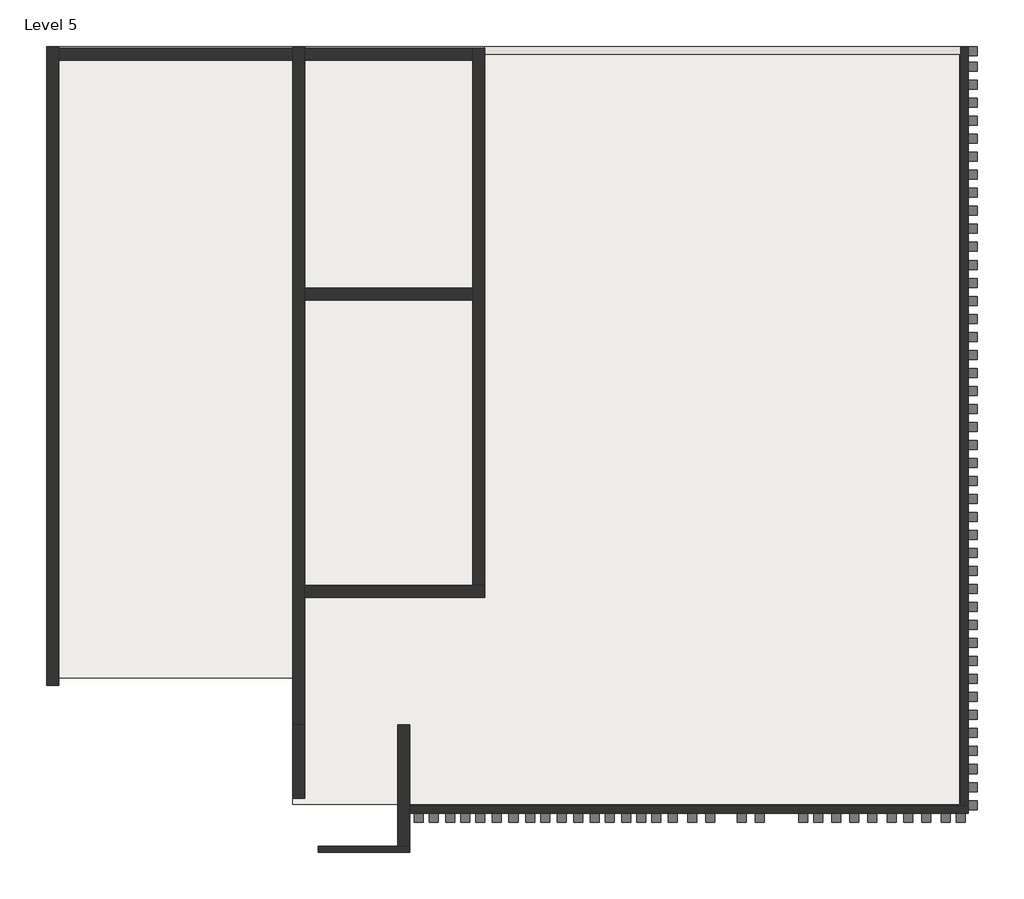
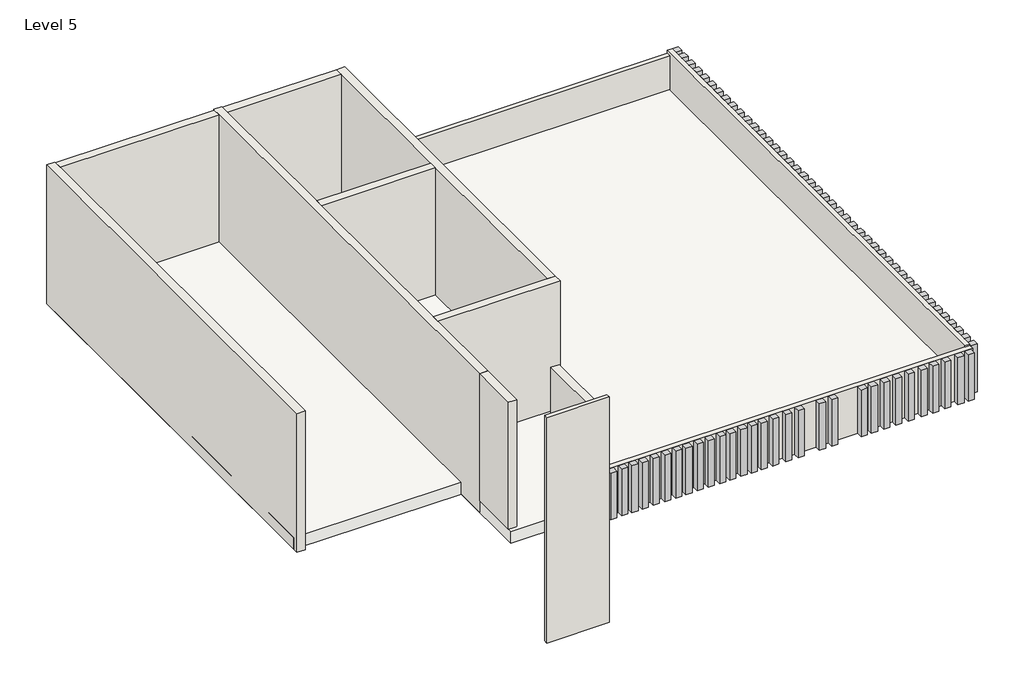
# One storey: 75 proxies, 12 walls, 1 roof.
"""IFC4 building model written with IfcOpenShell, lengths in millimetres."""

from ifc_helpers import new_model, si_unit, frame, origin, place, context, project, spatial, polyline, outline, extrude, faceted_brep, element, save

model = new_model("IFC4")

# Units and contexts
model_context = context("Model", 3, world=origin())
ifc_project = project(units=[si_unit("LENGTHUNIT", "METRE", prefix="MILLI")], contexts=[model_context])

# Site, building, storey
site = spatial("IfcSite", under=ifc_project)
building = spatial("IfcBuilding", under=site)
storey = spatial("IfcBuildingStorey", under=building, Name="Level 5", Elevation=14630.4)

# Proxies
placement = place(None, origin())
element("IfcBuildingElementProxy", 1, Name="Cornice", ObjectType="Cornice", at=placement, inside=storey, context=model_context, shape_type="SweptSolid", body=[
    extrude(outline(polyline([(-3003.9749149, -2254.9518013), (-3003.9749149, -2407.3518013), (-3156.3749149, -2407.3518013), (-3156.3749149, -2254.9518013), (-3003.9749149, -2254.9518013)])), frame((0.0, 0.0, 14630.4), z_axis=(0.0, 0.0, 1.0), x_axis=(1.0, 0.0, 0.0)), (0.0, 0.0, 1.0), 1229.0328786),
])
element("IfcBuildingElementProxy", 2, Name="Cornice", ObjectType="Cornice", at=placement, inside=storey, context=model_context, shape_type="SweptSolid", body=[
    extrude(outline(polyline([(-2749.9749149, -2254.9518013), (-2749.9749149, -2407.3518013), (-2902.3749149, -2407.3518013), (-2902.3749149, -2254.9518013), (-2749.9749149, -2254.9518013)])), frame((0.0, 0.0, 14630.4), z_axis=(0.0, 0.0, 1.0), x_axis=(1.0, 0.0, 0.0)), (0.0, 0.0, 1.0), 1229.0328786),
])
element("IfcBuildingElementProxy", 3, Name="Cornice", ObjectType="Cornice", at=placement, inside=storey, context=model_context, shape_type="SweptSolid", body=[
    extrude(outline(polyline([(-2470.5749149, -2254.9518013), (-2470.5749149, -2407.3518013), (-2622.9749149, -2407.3518013), (-2622.9749149, -2254.9518013), (-2470.5749149, -2254.9518013)])), frame((0.0, 0.0, 14630.4), z_axis=(0.0, 0.0, 1.0), x_axis=(1.0, 0.0, 0.0)), (0.0, 0.0, 1.0), 1229.0328786),
])
element("IfcBuildingElementProxy", 4, Name="Cornice", ObjectType="Cornice", at=placement, inside=storey, context=model_context, shape_type="SweptSolid", body=[
    extrude(outline(polyline([(-2216.5749149, -2254.9518013), (-2216.5749149, -2407.3518013), (-2368.9749149, -2407.3518013), (-2368.9749149, -2254.9518013), (-2216.5749149, -2254.9518013)])), frame((0.0, 0.0, 14630.4), z_axis=(0.0, 0.0, 1.0), x_axis=(1.0, 0.0, 0.0)), (0.0, 0.0, 1.0), 1229.0328786),
])
element("IfcBuildingElementProxy", 5, Name="Cornice", ObjectType="Cornice", at=placement, inside=storey, context=model_context, shape_type="SweptSolid", body=[
    extrude(outline(polyline([(-1962.5749149, -2254.9518013), (-1962.5749149, -2407.3518013), (-2114.9749149, -2407.3518013), (-2114.9749149, -2254.9518013), (-1962.5749149, -2254.9518013)])), frame((0.0, 0.0, 14630.4), z_axis=(0.0, 0.0, 1.0), x_axis=(1.0, 0.0, 0.0)), (0.0, 0.0, 1.0), 1229.0328786),
])
element("IfcBuildingElementProxy", 6, Name="Cornice", ObjectType="Cornice", at=placement, inside=storey, context=model_context, shape_type="SweptSolid", body=[
    extrude(outline(polyline([(-1683.1749149, -2254.9518013), (-1683.1749149, -2407.3518013), (-1835.5749149, -2407.3518013), (-1835.5749149, -2254.9518013), (-1683.1749149, -2254.9518013)])), frame((0.0, 0.0, 14630.4), z_axis=(0.0, 0.0, 1.0), x_axis=(1.0, 0.0, 0.0)), (0.0, 0.0, 1.0), 1229.0328786),
])
element("IfcBuildingElementProxy", 7, Name="Cornice", ObjectType="Cornice", at=placement, inside=storey, context=model_context, shape_type="SweptSolid", body=[
    extrude(outline(polyline([(-1403.7749149, -2254.9518013), (-1403.7749149, -2407.3518013), (-1556.1749149, -2407.3518013), (-1556.1749149, -2254.9518013), (-1403.7749149, -2254.9518013)])), frame((0.0, 0.0, 14630.4), z_axis=(0.0, 0.0, 1.0), x_axis=(1.0, 0.0, 0.0)), (0.0, 0.0, 1.0), 1229.0328786),
])
element("IfcBuildingElementProxy", 8, Name="Cornice", ObjectType="Cornice", at=placement, inside=storey, context=model_context, shape_type="SweptSolid", body=[
    extrude(outline(polyline([(-1124.3749149, -2254.9518013), (-1124.3749149, -2407.3518013), (-1276.7749149, -2407.3518013), (-1276.7749149, -2254.9518013), (-1124.3749149, -2254.9518013)])), frame((0.0, 0.0, 14630.4), z_axis=(0.0, 0.0, 1.0), x_axis=(1.0, 0.0, 0.0)), (0.0, 0.0, 1.0), 1229.0328786),
])
element("IfcBuildingElementProxy", 9, Name="Cornice", ObjectType="Cornice", at=placement, inside=storey, context=model_context, shape_type="SweptSolid", body=[
    extrude(outline(polyline([(-870.3749149, -2254.9518013), (-870.3749149, -2407.3518013), (-1022.7749149, -2407.3518013), (-1022.7749149, -2254.9518013), (-870.3749149, -2254.9518013)])), frame((0.0, 0.0, 14630.4), z_axis=(0.0, 0.0, 1.0), x_axis=(1.0, 0.0, 0.0)), (0.0, 0.0, 1.0), 1229.0328786),
])
element("IfcBuildingElementProxy", 10, Name="Cornice", ObjectType="Cornice", at=placement, inside=storey, context=model_context, shape_type="SweptSolid", body=[
    extrude(outline(polyline([(-590.9749149, -2254.9518013), (-590.9749149, -2407.3518013), (-743.3749149, -2407.3518013), (-743.3749149, -2254.9518013), (-590.9749149, -2254.9518013)])), frame((0.0, 0.0, 14630.4), z_axis=(0.0, 0.0, 1.0), x_axis=(1.0, 0.0, 0.0)), (0.0, 0.0, 1.0), 1229.0328786),
])
element("IfcBuildingElementProxy", 11, Name="Cornice", ObjectType="Cornice", at=placement, inside=storey, context=model_context, shape_type="SweptSolid", body=[
    extrude(outline(polyline([(-311.5749149, -2254.9518013), (-311.5749149, -2407.3518013), (-463.9749149, -2407.3518013), (-463.9749149, -2254.9518013), (-311.5749149, -2254.9518013)])), frame((0.0, 0.0, 14630.4), z_axis=(0.0, 0.0, 1.0), x_axis=(1.0, 0.0, 0.0)), (0.0, 0.0, 1.0), 1229.0328786),
])
element("IfcBuildingElementProxy", 12, Name="Cornice", ObjectType="Cornice", at=placement, inside=storey, context=model_context, shape_type="SweptSolid", body=[
    extrude(outline(polyline([(-32.1749149, -2254.9518013), (-32.1749149, -2407.3518013), (-184.5749149, -2407.3518013), (-184.5749149, -2254.9518013), (-32.1749149, -2254.9518013)])), frame((0.0, 0.0, 14630.4), z_axis=(0.0, 0.0, 1.0), x_axis=(1.0, 0.0, 0.0)), (0.0, 0.0, 1.0), 1229.0328786),
])
element("IfcBuildingElementProxy", 13, Name="Cornice", ObjectType="Cornice", at=placement, inside=storey, context=model_context, shape_type="SweptSolid", body=[
    extrude(outline(polyline([(221.8250851, -2254.9518013), (221.8250851, -2407.3518013), (69.4250851, -2407.3518013), (69.4250851, -2254.9518013), (221.8250851, -2254.9518013)])), frame((0.0, 0.0, 14630.4), z_axis=(0.0, 0.0, 1.0), x_axis=(1.0, 0.0, 0.0)), (0.0, 0.0, 1.0), 1229.0328786),
])
element("IfcBuildingElementProxy", 14, Name="Cornice", ObjectType="Cornice", at=placement, inside=storey, context=model_context, shape_type="SweptSolid", body=[
    extrude(outline(polyline([(501.2250851, -2254.9518013), (501.2250851, -2407.3518013), (348.8250851, -2407.3518013), (348.8250851, -2254.9518013), (501.2250851, -2254.9518013)])), frame((0.0, 0.0, 14630.4), z_axis=(0.0, 0.0, 1.0), x_axis=(1.0, 0.0, 0.0)), (0.0, 0.0, 1.0), 1229.0328786),
])
element("IfcBuildingElementProxy", 15, Name="Cornice", ObjectType="Cornice", at=placement, inside=storey, context=model_context, shape_type="SweptSolid", body=[
    extrude(outline(polyline([(755.2250851, -2254.9518013), (755.2250851, -2407.3518013), (602.8250851, -2407.3518013), (602.8250851, -2254.9518013), (755.2250851, -2254.9518013)])), frame((0.0, 0.0, 14630.4), z_axis=(0.0, 0.0, 1.0), x_axis=(1.0, 0.0, 0.0)), (0.0, 0.0, 1.0), 1229.0328786),
])
element("IfcBuildingElementProxy", 16, Name="Cornice", ObjectType="Cornice", at=placement, inside=storey, context=model_context, shape_type="SweptSolid", body=[
    extrude(outline(polyline([(1009.2250851, -2254.9518013), (1009.2250851, -2407.3518013), (856.8250851, -2407.3518013), (856.8250851, -2254.9518013), (1009.2250851, -2254.9518013)])), frame((0.0, 0.0, 14630.4), z_axis=(0.0, 0.0, 1.0), x_axis=(1.0, 0.0, 0.0)), (0.0, 0.0, 1.0), 1229.0328786),
])
element("IfcBuildingElementProxy", 17, Name="Cornice", ObjectType="Cornice", at=placement, inside=storey, context=model_context, shape_type="SweptSolid", body=[
    extrude(outline(polyline([(1288.6250851, -2254.9518013), (1288.6250851, -2407.3518013), (1136.2250851, -2407.3518013), (1136.2250851, -2254.9518013), (1288.6250851, -2254.9518013)])), frame((0.0, 0.0, 14630.4), z_axis=(0.0, 0.0, 1.0), x_axis=(1.0, 0.0, 0.0)), (0.0, 0.0, 1.0), 1229.0328786),
])
element("IfcBuildingElementProxy", 18, Name="Cornice", ObjectType="Cornice", at=placement, inside=storey, context=model_context, shape_type="SweptSolid", body=[
    extrude(outline(polyline([(1618.8250851, -2254.9518013), (1618.8250851, -2407.3518013), (1466.4250851, -2407.3518013), (1466.4250851, -2254.9518013), (1618.8250851, -2254.9518013)])), frame((0.0, 0.0, 14630.4), z_axis=(0.0, 0.0, 1.0), x_axis=(1.0, 0.0, 0.0)), (0.0, 0.0, 1.0), 1229.0328786),
])
element("IfcBuildingElementProxy", 19, Name="Cornice", ObjectType="Cornice", at=placement, inside=storey, context=model_context, shape_type="SweptSolid", body=[
    extrude(outline(polyline([(1923.6250851, -2254.9518013), (1923.6250851, -2407.3518013), (1771.2250851, -2407.3518013), (1771.2250851, -2254.9518013), (1923.6250851, -2254.9518013)])), frame((0.0, 0.0, 14630.4), z_axis=(0.0, 0.0, 1.0), x_axis=(1.0, 0.0, 0.0)), (0.0, 0.0, 1.0), 1229.0328786),
])
element("IfcBuildingElementProxy", 20, Name="Cornice", ObjectType="Cornice", at=placement, inside=storey, context=model_context, shape_type="SweptSolid", body=[
    extrude(outline(polyline([(2457.0250851, -2254.9518013), (2457.0250851, -2407.3518013), (2304.6250851, -2407.3518013), (2304.6250851, -2254.9518013), (2457.0250851, -2254.9518013)])), frame((0.0, 0.0, 14630.4), z_axis=(0.0, 0.0, 1.0), x_axis=(1.0, 0.0, 0.0)), (0.0, 0.0, 1.0), 1229.0328786),
])
element("IfcBuildingElementProxy", 21, Name="Cornice", ObjectType="Cornice", at=placement, inside=storey, context=model_context, shape_type="SweptSolid", body=[
    extrude(outline(polyline([(2761.8250851, -2254.9518013), (2761.8250851, -2407.3518013), (2609.4250851, -2407.3518013), (2609.4250851, -2254.9518013), (2761.8250851, -2254.9518013)])), frame((0.0, 0.0, 14630.4), z_axis=(0.0, 0.0, 1.0), x_axis=(1.0, 0.0, 0.0)), (0.0, 0.0, 1.0), 1229.0328786),
])
element("IfcBuildingElementProxy", 22, Name="Cornice", ObjectType="Cornice", at=placement, inside=storey, context=model_context, shape_type="SweptSolid", body=[
    extrude(outline(polyline([(3498.4250851, -2254.9518013), (3498.4250851, -2407.3518013), (3346.0250851, -2407.3518013), (3346.0250851, -2254.9518013), (3498.4250851, -2254.9518013)])), frame((0.0, 0.0, 14630.4), z_axis=(0.0, 0.0, 1.0), x_axis=(1.0, 0.0, 0.0)), (0.0, 0.0, 1.0), 1229.0328786),
])
element("IfcBuildingElementProxy", 23, Name="Cornice", ObjectType="Cornice", at=placement, inside=storey, context=model_context, shape_type="SweptSolid", body=[
    extrude(outline(polyline([(3752.4250851, -2254.9518013), (3752.4250851, -2407.3518013), (3600.0250851, -2407.3518013), (3600.0250851, -2254.9518013), (3752.4250851, -2254.9518013)])), frame((0.0, 0.0, 14630.4), z_axis=(0.0, 0.0, 1.0), x_axis=(1.0, 0.0, 0.0)), (0.0, 0.0, 1.0), 1229.0328786),
])
element("IfcBuildingElementProxy", 24, Name="Cornice", ObjectType="Cornice", at=placement, inside=storey, context=model_context, shape_type="SweptSolid", body=[
    extrude(outline(polyline([(4057.2250851, -2254.9518013), (4057.2250851, -2407.3518013), (3904.8250851, -2407.3518013), (3904.8250851, -2254.9518013), (4057.2250851, -2254.9518013)])), frame((0.0, 0.0, 14630.4), z_axis=(0.0, 0.0, 1.0), x_axis=(1.0, 0.0, 0.0)), (0.0, 0.0, 1.0), 1229.0328786),
])
element("IfcBuildingElementProxy", 25, Name="Cornice", ObjectType="Cornice", at=placement, inside=storey, context=model_context, shape_type="SweptSolid", body=[
    extrude(outline(polyline([(4362.0250851, -2254.9518013), (4362.0250851, -2407.3518013), (4209.6250851, -2407.3518013), (4209.6250851, -2254.9518013), (4362.0250851, -2254.9518013)])), frame((0.0, 0.0, 14630.4), z_axis=(0.0, 0.0, 1.0), x_axis=(1.0, 0.0, 0.0)), (0.0, 0.0, 1.0), 1229.0328786),
])
element("IfcBuildingElementProxy", 26, Name="Cornice", ObjectType="Cornice", at=placement, inside=storey, context=model_context, shape_type="SweptSolid", body=[
    extrude(outline(polyline([(4666.8250851, -2254.9518013), (4666.8250851, -2407.3518013), (4514.4250851, -2407.3518013), (4514.4250851, -2254.9518013), (4666.8250851, -2254.9518013)])), frame((0.0, 0.0, 14630.4), z_axis=(0.0, 0.0, 1.0), x_axis=(1.0, 0.0, 0.0)), (0.0, 0.0, 1.0), 1229.0328786),
])
element("IfcBuildingElementProxy", 27, Name="Cornice", ObjectType="Cornice", at=placement, inside=storey, context=model_context, shape_type="SweptSolid", body=[
    extrude(outline(polyline([(4997.0250851, -2254.9518013), (4997.0250851, -2407.3518013), (4844.6250851, -2407.3518013), (4844.6250851, -2254.9518013), (4997.0250851, -2254.9518013)])), frame((0.0, 0.0, 14630.4), z_axis=(0.0, 0.0, 1.0), x_axis=(1.0, 0.0, 0.0)), (0.0, 0.0, 1.0), 1229.0328786),
])
element("IfcBuildingElementProxy", 28, Name="Cornice", ObjectType="Cornice", at=placement, inside=storey, context=model_context, shape_type="SweptSolid", body=[
    extrude(outline(polyline([(5276.4250851, -2254.9518013), (5276.4250851, -2407.3518013), (5124.0250851, -2407.3518013), (5124.0250851, -2254.9518013), (5276.4250851, -2254.9518013)])), frame((0.0, 0.0, 14630.4), z_axis=(0.0, 0.0, 1.0), x_axis=(1.0, 0.0, 0.0)), (0.0, 0.0, 1.0), 1229.0328786),
])
element("IfcBuildingElementProxy", 29, Name="Cornice", ObjectType="Cornice", at=placement, inside=storey, context=model_context, shape_type="SweptSolid", body=[
    extrude(outline(polyline([(5581.2250851, -2254.9518013), (5581.2250851, -2407.3518013), (5428.8250851, -2407.3518013), (5428.8250851, -2254.9518013), (5581.2250851, -2254.9518013)])), frame((0.0, 0.0, 14630.4), z_axis=(0.0, 0.0, 1.0), x_axis=(1.0, 0.0, 0.0)), (0.0, 0.0, 1.0), 1229.0328786),
])
element("IfcBuildingElementProxy", 30, Name="Cornice", ObjectType="Cornice", at=placement, inside=storey, context=model_context, shape_type="SweptSolid", body=[
    extrude(outline(polyline([(5911.4250851, -2254.9518013), (5911.4250851, -2407.3518013), (5759.0250851, -2407.3518013), (5759.0250851, -2254.9518013), (5911.4250851, -2254.9518013)])), frame((0.0, 0.0, 14630.4), z_axis=(0.0, 0.0, 1.0), x_axis=(1.0, 0.0, 0.0)), (0.0, 0.0, 1.0), 1229.0328786),
])
element("IfcBuildingElementProxy", 31, Name="Cornice", ObjectType="Cornice", at=placement, inside=storey, context=model_context, shape_type="SweptSolid", body=[
    extrude(outline(polyline([(6165.4250851, -2254.9518013), (6165.4250851, -2407.3518013), (6013.0250851, -2407.3518013), (6013.0250851, -2254.9518013), (6165.4250851, -2254.9518013)])), frame((0.0, 0.0, 14630.4), z_axis=(0.0, 0.0, 1.0), x_axis=(1.0, 0.0, 0.0)), (0.0, 0.0, 1.0), 1229.0328786),
])
element("IfcBuildingElementProxy", 32, Name="Cornice", ObjectType="Cornice", at=placement, inside=storey, context=model_context, shape_type="SweptSolid", body=[
    extrude(outline(polyline([(6216.2250851, -2039.0518013), (6368.6250851, -2039.0518013), (6368.6250851, -2191.4518013), (6216.2250851, -2191.4518013), (6216.2250851, -2039.0518013)])), frame((0.0, 0.0, 14630.4), z_axis=(0.0, 0.0, 1.0), x_axis=(1.0, 0.0, 0.0)), (0.0, 0.0, 1.0), 1259.5551035),
])
element("IfcBuildingElementProxy", 33, Name="Cornice", ObjectType="Cornice", at=placement, inside=storey, context=model_context, shape_type="SweptSolid", body=[
    extrude(outline(polyline([(6216.2250851, -1734.2518013), (6368.6250851, -1734.2518013), (6368.6250851, -1886.6518013), (6216.2250851, -1886.6518013), (6216.2250851, -1734.2518013)])), frame((0.0, 0.0, 14630.4), z_axis=(0.0, 0.0, 1.0), x_axis=(1.0, 0.0, 0.0)), (0.0, 0.0, 1.0), 1259.5551035),
])
element("IfcBuildingElementProxy", 34, Name="Cornice", ObjectType="Cornice", at=placement, inside=storey, context=model_context, shape_type="SweptSolid", body=[
    extrude(outline(polyline([(6216.2250851, -1429.4518013), (6368.6250851, -1429.4518013), (6368.6250851, -1581.8518013), (6216.2250851, -1581.8518013), (6216.2250851, -1429.4518013)])), frame((0.0, 0.0, 14630.4), z_axis=(0.0, 0.0, 1.0), x_axis=(1.0, 0.0, 0.0)), (0.0, 0.0, 1.0), 1259.5551035),
])
element("IfcBuildingElementProxy", 35, Name="Cornice", ObjectType="Cornice", at=placement, inside=storey, context=model_context, shape_type="SweptSolid", body=[
    extrude(outline(polyline([(6216.2250851, -1124.6518013), (6368.6250851, -1124.6518013), (6368.6250851, -1277.0518013), (6216.2250851, -1277.0518013), (6216.2250851, -1124.6518013)])), frame((0.0, 0.0, 14630.4), z_axis=(0.0, 0.0, 1.0), x_axis=(1.0, 0.0, 0.0)), (0.0, 0.0, 1.0), 1259.5551035),
])
element("IfcBuildingElementProxy", 36, Name="Cornice", ObjectType="Cornice", at=placement, inside=storey, context=model_context, shape_type="SweptSolid", body=[
    extrude(outline(polyline([(6216.2250851, -819.8518013), (6368.6250851, -819.8518013), (6368.6250851, -972.2518013), (6216.2250851, -972.2518013), (6216.2250851, -819.8518013)])), frame((0.0, 0.0, 14630.4), z_axis=(0.0, 0.0, 1.0), x_axis=(1.0, 0.0, 0.0)), (0.0, 0.0, 1.0), 1259.5551035),
])
element("IfcBuildingElementProxy", 37, Name="Cornice", ObjectType="Cornice", at=placement, inside=storey, context=model_context, shape_type="SweptSolid", body=[
    extrude(outline(polyline([(6216.2250851, -515.0518013), (6368.6250851, -515.0518013), (6368.6250851, -667.4518013), (6216.2250851, -667.4518013), (6216.2250851, -515.0518013)])), frame((0.0, 0.0, 14630.4), z_axis=(0.0, 0.0, 1.0), x_axis=(1.0, 0.0, 0.0)), (0.0, 0.0, 1.0), 1259.5551035),
])
element("IfcBuildingElementProxy", 38, Name="Cornice", ObjectType="Cornice", at=placement, inside=storey, context=model_context, shape_type="SweptSolid", body=[
    extrude(outline(polyline([(6216.2250851, -210.2518013), (6368.6250851, -210.2518013), (6368.6250851, -362.6518013), (6216.2250851, -362.6518013), (6216.2250851, -210.2518013)])), frame((0.0, 0.0, 14630.4), z_axis=(0.0, 0.0, 1.0), x_axis=(1.0, 0.0, 0.0)), (0.0, 0.0, 1.0), 1259.5551035),
])
element("IfcBuildingElementProxy", 39, Name="Cornice", ObjectType="Cornice", at=placement, inside=storey, context=model_context, shape_type="SweptSolid", body=[
    extrude(outline(polyline([(6216.2250851, 94.5481987), (6368.6250851, 94.5481987), (6368.6250851, -57.8518013), (6216.2250851, -57.8518013), (6216.2250851, 94.5481987)])), frame((0.0, 0.0, 14630.4), z_axis=(0.0, 0.0, 1.0), x_axis=(1.0, 0.0, 0.0)), (0.0, 0.0, 1.0), 1259.5551035),
])
element("IfcBuildingElementProxy", 40, Name="Cornice", ObjectType="Cornice", at=placement, inside=storey, context=model_context, shape_type="SweptSolid", body=[
    extrude(outline(polyline([(6216.2250851, 399.3481987), (6368.6250851, 399.3481987), (6368.6250851, 246.9481987), (6216.2250851, 246.9481987), (6216.2250851, 399.3481987)])), frame((0.0, 0.0, 14630.4), z_axis=(0.0, 0.0, 1.0), x_axis=(1.0, 0.0, 0.0)), (0.0, 0.0, 1.0), 1259.5551035),
])
element("IfcBuildingElementProxy", 41, Name="Cornice", ObjectType="Cornice", at=placement, inside=storey, context=model_context, shape_type="SweptSolid", body=[
    extrude(outline(polyline([(6216.2250851, 704.1481987), (6368.6250851, 704.1481987), (6368.6250851, 551.7481987), (6216.2250851, 551.7481987), (6216.2250851, 704.1481987)])), frame((0.0, 0.0, 14630.4), z_axis=(0.0, 0.0, 1.0), x_axis=(1.0, 0.0, 0.0)), (0.0, 0.0, 1.0), 1259.5551035),
])
element("IfcBuildingElementProxy", 42, Name="Cornice", ObjectType="Cornice", at=placement, inside=storey, context=model_context, shape_type="SweptSolid", body=[
    extrude(outline(polyline([(6216.2250851, 1008.9481987), (6368.6250851, 1008.9481987), (6368.6250851, 856.5481987), (6216.2250851, 856.5481987), (6216.2250851, 1008.9481987)])), frame((0.0, 0.0, 14630.4), z_axis=(0.0, 0.0, 1.0), x_axis=(1.0, 0.0, 0.0)), (0.0, 0.0, 1.0), 1259.5551035),
])
element("IfcBuildingElementProxy", 43, Name="Cornice", ObjectType="Cornice", at=placement, inside=storey, context=model_context, shape_type="SweptSolid", body=[
    extrude(outline(polyline([(6216.2250851, 1313.7481987), (6368.6250851, 1313.7481987), (6368.6250851, 1161.3481987), (6216.2250851, 1161.3481987), (6216.2250851, 1313.7481987)])), frame((0.0, 0.0, 14630.4), z_axis=(0.0, 0.0, 1.0), x_axis=(1.0, 0.0, 0.0)), (0.0, 0.0, 1.0), 1259.5551035),
])
element("IfcBuildingElementProxy", 44, Name="Cornice", ObjectType="Cornice", at=placement, inside=storey, context=model_context, shape_type="SweptSolid", body=[
    extrude(outline(polyline([(6216.2250851, 1618.5481987), (6368.6250851, 1618.5481987), (6368.6250851, 1466.1481987), (6216.2250851, 1466.1481987), (6216.2250851, 1618.5481987)])), frame((0.0, 0.0, 14630.4), z_axis=(0.0, 0.0, 1.0), x_axis=(1.0, 0.0, 0.0)), (0.0, 0.0, 1.0), 1259.5551035),
])
element("IfcBuildingElementProxy", 45, Name="Cornice", ObjectType="Cornice", at=placement, inside=storey, context=model_context, shape_type="SweptSolid", body=[
    extrude(outline(polyline([(6216.2250851, 1923.3481987), (6368.6250851, 1923.3481987), (6368.6250851, 1770.9481987), (6216.2250851, 1770.9481987), (6216.2250851, 1923.3481987)])), frame((0.0, 0.0, 14630.4), z_axis=(0.0, 0.0, 1.0), x_axis=(1.0, 0.0, 0.0)), (0.0, 0.0, 1.0), 1259.5551035),
])
element("IfcBuildingElementProxy", 46, Name="Cornice", ObjectType="Cornice", at=placement, inside=storey, context=model_context, shape_type="SweptSolid", body=[
    extrude(outline(polyline([(6216.2250851, 2228.1481987), (6368.6250851, 2228.1481987), (6368.6250851, 2075.7481987), (6216.2250851, 2075.7481987), (6216.2250851, 2228.1481987)])), frame((0.0, 0.0, 14630.4), z_axis=(0.0, 0.0, 1.0), x_axis=(1.0, 0.0, 0.0)), (0.0, 0.0, 1.0), 1259.5551035),
])
element("IfcBuildingElementProxy", 47, Name="Cornice", ObjectType="Cornice", at=placement, inside=storey, context=model_context, shape_type="SweptSolid", body=[
    extrude(outline(polyline([(6216.2250851, 2532.9481987), (6368.6250851, 2532.9481987), (6368.6250851, 2380.5481987), (6216.2250851, 2380.5481987), (6216.2250851, 2532.9481987)])), frame((0.0, 0.0, 14630.4), z_axis=(0.0, 0.0, 1.0), x_axis=(1.0, 0.0, 0.0)), (0.0, 0.0, 1.0), 1259.5551035),
])
element("IfcBuildingElementProxy", 48, Name="Cornice", ObjectType="Cornice", at=placement, inside=storey, context=model_context, shape_type="SweptSolid", body=[
    extrude(outline(polyline([(6216.2250851, 2837.7481987), (6368.6250851, 2837.7481987), (6368.6250851, 2685.3481987), (6216.2250851, 2685.3481987), (6216.2250851, 2837.7481987)])), frame((0.0, 0.0, 14630.4), z_axis=(0.0, 0.0, 1.0), x_axis=(1.0, 0.0, 0.0)), (0.0, 0.0, 1.0), 1259.5551035),
])
element("IfcBuildingElementProxy", 49, Name="Cornice", ObjectType="Cornice", at=placement, inside=storey, context=model_context, shape_type="SweptSolid", body=[
    extrude(outline(polyline([(6216.2250851, 3142.5481987), (6368.6250851, 3142.5481987), (6368.6250851, 2990.1481987), (6216.2250851, 2990.1481987), (6216.2250851, 3142.5481987)])), frame((0.0, 0.0, 14630.4), z_axis=(0.0, 0.0, 1.0), x_axis=(1.0, 0.0, 0.0)), (0.0, 0.0, 1.0), 1259.5551035),
])
element("IfcBuildingElementProxy", 50, Name="Cornice", ObjectType="Cornice", at=placement, inside=storey, context=model_context, shape_type="SweptSolid", body=[
    extrude(outline(polyline([(6216.2250851, 3447.3481987), (6368.6250851, 3447.3481987), (6368.6250851, 3294.9481987), (6216.2250851, 3294.9481987), (6216.2250851, 3447.3481987)])), frame((0.0, 0.0, 14630.4), z_axis=(0.0, 0.0, 1.0), x_axis=(1.0, 0.0, 0.0)), (0.0, 0.0, 1.0), 1259.5551035),
])
element("IfcBuildingElementProxy", 51, Name="Cornice", ObjectType="Cornice", at=placement, inside=storey, context=model_context, shape_type="SweptSolid", body=[
    extrude(outline(polyline([(6216.2250851, 3447.3481987), (6368.6250851, 3447.3481987), (6368.6250851, 3294.9481987), (6216.2250851, 3294.9481987), (6216.2250851, 3447.3481987)])), frame((0.0, 0.0, 14630.4), z_axis=(0.0, 0.0, 1.0), x_axis=(1.0, 0.0, 0.0)), (0.0, 0.0, 1.0), 1259.5551035),
])
element("IfcBuildingElementProxy", 52, Name="Cornice", ObjectType="Cornice", at=placement, inside=storey, context=model_context, shape_type="SweptSolid", body=[
    extrude(outline(polyline([(6216.2250851, 3752.1481987), (6368.6250851, 3752.1481987), (6368.6250851, 3599.7481987), (6216.2250851, 3599.7481987), (6216.2250851, 3752.1481987)])), frame((0.0, 0.0, 14630.4), z_axis=(0.0, 0.0, 1.0), x_axis=(1.0, 0.0, 0.0)), (0.0, 0.0, 1.0), 1259.5551035),
])
element("IfcBuildingElementProxy", 53, Name="Cornice", ObjectType="Cornice", at=placement, inside=storey, context=model_context, shape_type="SweptSolid", body=[
    extrude(outline(polyline([(6216.2250851, 4056.9481987), (6368.6250851, 4056.9481987), (6368.6250851, 3904.5481987), (6216.2250851, 3904.5481987), (6216.2250851, 4056.9481987)])), frame((0.0, 0.0, 14630.4), z_axis=(0.0, 0.0, 1.0), x_axis=(1.0, 0.0, 0.0)), (0.0, 0.0, 1.0), 1259.5551035),
])
element("IfcBuildingElementProxy", 54, Name="Cornice", ObjectType="Cornice", at=placement, inside=storey, context=model_context, shape_type="SweptSolid", body=[
    extrude(outline(polyline([(6216.2250851, 4361.7481987), (6368.6250851, 4361.7481987), (6368.6250851, 4209.3481987), (6216.2250851, 4209.3481987), (6216.2250851, 4361.7481987)])), frame((0.0, 0.0, 14630.4), z_axis=(0.0, 0.0, 1.0), x_axis=(1.0, 0.0, 0.0)), (0.0, 0.0, 1.0), 1259.5551035),
])
element("IfcBuildingElementProxy", 55, Name="Cornice", ObjectType="Cornice", at=placement, inside=storey, context=model_context, shape_type="SweptSolid", body=[
    extrude(outline(polyline([(6216.2250851, 4666.5481987), (6368.6250851, 4666.5481987), (6368.6250851, 4514.1481987), (6216.2250851, 4514.1481987), (6216.2250851, 4666.5481987)])), frame((0.0, 0.0, 14630.4), z_axis=(0.0, 0.0, 1.0), x_axis=(1.0, 0.0, 0.0)), (0.0, 0.0, 1.0), 1259.5551035),
])
element("IfcBuildingElementProxy", 56, Name="Cornice", ObjectType="Cornice", at=placement, inside=storey, context=model_context, shape_type="SweptSolid", body=[
    extrude(outline(polyline([(6216.2250851, 4971.3481987), (6368.6250851, 4971.3481987), (6368.6250851, 4818.9481987), (6216.2250851, 4818.9481987), (6216.2250851, 4971.3481987)])), frame((0.0, 0.0, 14630.4), z_axis=(0.0, 0.0, 1.0), x_axis=(1.0, 0.0, 0.0)), (0.0, 0.0, 1.0), 1259.5551035),
])
element("IfcBuildingElementProxy", 57, Name="Cornice", ObjectType="Cornice", at=placement, inside=storey, context=model_context, shape_type="SweptSolid", body=[
    extrude(outline(polyline([(6216.2250851, 5276.1481987), (6368.6250851, 5276.1481987), (6368.6250851, 5123.7481987), (6216.2250851, 5123.7481987), (6216.2250851, 5276.1481987)])), frame((0.0, 0.0, 14630.4), z_axis=(0.0, 0.0, 1.0), x_axis=(1.0, 0.0, 0.0)), (0.0, 0.0, 1.0), 1259.5551035),
])
element("IfcBuildingElementProxy", 58, Name="Cornice", ObjectType="Cornice", at=placement, inside=storey, context=model_context, shape_type="SweptSolid", body=[
    extrude(outline(polyline([(6216.2250851, 5580.9481987), (6368.6250851, 5580.9481987), (6368.6250851, 5428.5481987), (6216.2250851, 5428.5481987), (6216.2250851, 5580.9481987)])), frame((0.0, 0.0, 14630.4), z_axis=(0.0, 0.0, 1.0), x_axis=(1.0, 0.0, 0.0)), (0.0, 0.0, 1.0), 1259.5551035),
])
element("IfcBuildingElementProxy", 59, Name="Cornice", ObjectType="Cornice", at=placement, inside=storey, context=model_context, shape_type="SweptSolid", body=[
    extrude(outline(polyline([(6216.2250851, 5885.7481987), (6368.6250851, 5885.7481987), (6368.6250851, 5733.3481987), (6216.2250851, 5733.3481987), (6216.2250851, 5885.7481987)])), frame((0.0, 0.0, 14630.4), z_axis=(0.0, 0.0, 1.0), x_axis=(1.0, 0.0, 0.0)), (0.0, 0.0, 1.0), 1259.5551035),
])
element("IfcBuildingElementProxy", 60, Name="Cornice", ObjectType="Cornice", at=placement, inside=storey, context=model_context, shape_type="SweptSolid", body=[
    extrude(outline(polyline([(6216.2250851, 6190.5481987), (6368.6250851, 6190.5481987), (6368.6250851, 6038.1481987), (6216.2250851, 6038.1481987), (6216.2250851, 6190.5481987)])), frame((0.0, 0.0, 14630.4), z_axis=(0.0, 0.0, 1.0), x_axis=(1.0, 0.0, 0.0)), (0.0, 0.0, 1.0), 1259.5551035),
])
element("IfcBuildingElementProxy", 61, Name="Cornice", ObjectType="Cornice", at=placement, inside=storey, context=model_context, shape_type="SweptSolid", body=[
    extrude(outline(polyline([(6216.2250851, 6495.3481987), (6368.6250851, 6495.3481987), (6368.6250851, 6342.9481987), (6216.2250851, 6342.9481987), (6216.2250851, 6495.3481987)])), frame((0.0, 0.0, 14630.4), z_axis=(0.0, 0.0, 1.0), x_axis=(1.0, 0.0, 0.0)), (0.0, 0.0, 1.0), 1259.5551035),
])
element("IfcBuildingElementProxy", 62, Name="Cornice", ObjectType="Cornice", at=placement, inside=storey, context=model_context, shape_type="SweptSolid", body=[
    extrude(outline(polyline([(6216.2250851, 6800.1481987), (6368.6250851, 6800.1481987), (6368.6250851, 6647.7481987), (6216.2250851, 6647.7481987), (6216.2250851, 6800.1481987)])), frame((0.0, 0.0, 14630.4), z_axis=(0.0, 0.0, 1.0), x_axis=(1.0, 0.0, 0.0)), (0.0, 0.0, 1.0), 1259.5551035),
])
element("IfcBuildingElementProxy", 63, Name="Cornice", ObjectType="Cornice", at=placement, inside=storey, context=model_context, shape_type="SweptSolid", body=[
    extrude(outline(polyline([(6216.2250851, 7104.9481987), (6368.6250851, 7104.9481987), (6368.6250851, 6952.5481987), (6216.2250851, 6952.5481987), (6216.2250851, 7104.9481987)])), frame((0.0, 0.0, 14630.4), z_axis=(0.0, 0.0, 1.0), x_axis=(1.0, 0.0, 0.0)), (0.0, 0.0, 1.0), 1259.5551035),
])
element("IfcBuildingElementProxy", 64, Name="Cornice", ObjectType="Cornice", at=placement, inside=storey, context=model_context, shape_type="SweptSolid", body=[
    extrude(outline(polyline([(6216.2250851, 7409.7481987), (6368.6250851, 7409.7481987), (6368.6250851, 7257.3481987), (6216.2250851, 7257.3481987), (6216.2250851, 7409.7481987)])), frame((0.0, 0.0, 14630.4), z_axis=(0.0, 0.0, 1.0), x_axis=(1.0, 0.0, 0.0)), (0.0, 0.0, 1.0), 1259.5551035),
])
element("IfcBuildingElementProxy", 65, Name="Cornice", ObjectType="Cornice", at=placement, inside=storey, context=model_context, shape_type="SweptSolid", body=[
    extrude(outline(polyline([(6216.2250851, 7714.5481987), (6368.6250851, 7714.5481987), (6368.6250851, 7562.1481987), (6216.2250851, 7562.1481987), (6216.2250851, 7714.5481987)])), frame((0.0, 0.0, 14630.4), z_axis=(0.0, 0.0, 1.0), x_axis=(1.0, 0.0, 0.0)), (0.0, 0.0, 1.0), 1259.5551035),
])
element("IfcBuildingElementProxy", 66, Name="Cornice", ObjectType="Cornice", at=placement, inside=storey, context=model_context, shape_type="SweptSolid", body=[
    extrude(outline(polyline([(6216.2250851, 8019.3481987), (6368.6250851, 8019.3481987), (6368.6250851, 7866.9481987), (6216.2250851, 7866.9481987), (6216.2250851, 8019.3481987)])), frame((0.0, 0.0, 14630.4), z_axis=(0.0, 0.0, 1.0), x_axis=(1.0, 0.0, 0.0)), (0.0, 0.0, 1.0), 1259.5551035),
])
element("IfcBuildingElementProxy", 67, Name="Cornice", ObjectType="Cornice", at=placement, inside=storey, context=model_context, shape_type="SweptSolid", body=[
    extrude(outline(polyline([(6216.2250851, 8324.1481987), (6368.6250851, 8324.1481987), (6368.6250851, 8171.7481987), (6216.2250851, 8171.7481987), (6216.2250851, 8324.1481987)])), frame((0.0, 0.0, 14630.4), z_axis=(0.0, 0.0, 1.0), x_axis=(1.0, 0.0, 0.0)), (0.0, 0.0, 1.0), 1259.5551035),
])
element("IfcBuildingElementProxy", 68, Name="Cornice", ObjectType="Cornice", at=placement, inside=storey, context=model_context, shape_type="SweptSolid", body=[
    extrude(outline(polyline([(6216.2250851, 8628.9481987), (6368.6250851, 8628.9481987), (6368.6250851, 8476.5481987), (6216.2250851, 8476.5481987), (6216.2250851, 8628.9481987)])), frame((0.0, 0.0, 14630.4), z_axis=(0.0, 0.0, 1.0), x_axis=(1.0, 0.0, 0.0)), (0.0, 0.0, 1.0), 1259.5551035),
])
element("IfcBuildingElementProxy", 69, Name="Cornice", ObjectType="Cornice", at=placement, inside=storey, context=model_context, shape_type="SweptSolid", body=[
    extrude(outline(polyline([(6216.2250851, 8933.7481987), (6368.6250851, 8933.7481987), (6368.6250851, 8781.3481987), (6216.2250851, 8781.3481987), (6216.2250851, 8933.7481987)])), frame((0.0, 0.0, 14630.4), z_axis=(0.0, 0.0, 1.0), x_axis=(1.0, 0.0, 0.0)), (0.0, 0.0, 1.0), 1259.5551035),
])
element("IfcBuildingElementProxy", 70, Name="Cornice", ObjectType="Cornice", at=placement, inside=storey, context=model_context, shape_type="SweptSolid", body=[
    extrude(outline(polyline([(6216.2250851, 9238.5481987), (6368.6250851, 9238.5481987), (6368.6250851, 9086.1481987), (6216.2250851, 9086.1481987), (6216.2250851, 9238.5481987)])), frame((0.0, 0.0, 14630.4), z_axis=(0.0, 0.0, 1.0), x_axis=(1.0, 0.0, 0.0)), (0.0, 0.0, 1.0), 1259.5551035),
])
element("IfcBuildingElementProxy", 71, Name="Cornice", ObjectType="Cornice", at=placement, inside=storey, context=model_context, shape_type="SweptSolid", body=[
    extrude(outline(polyline([(6216.2250851, 9543.3481987), (6368.6250851, 9543.3481987), (6368.6250851, 9390.9481987), (6216.2250851, 9390.9481987), (6216.2250851, 9543.3481987)])), frame((0.0, 0.0, 14630.4), z_axis=(0.0, 0.0, 1.0), x_axis=(1.0, 0.0, 0.0)), (0.0, 0.0, 1.0), 1259.5551035),
])
element("IfcBuildingElementProxy", 72, Name="Cornice", ObjectType="Cornice", at=placement, inside=storey, context=model_context, shape_type="SweptSolid", body=[
    extrude(outline(polyline([(6216.2250851, 9848.1481987), (6368.6250851, 9848.1481987), (6368.6250851, 9695.7481987), (6216.2250851, 9695.7481987), (6216.2250851, 9848.1481987)])), frame((0.0, 0.0, 14630.4), z_axis=(0.0, 0.0, 1.0), x_axis=(1.0, 0.0, 0.0)), (0.0, 0.0, 1.0), 1259.5551035),
])
element("IfcBuildingElementProxy", 73, Name="Cornice", ObjectType="Cornice", at=placement, inside=storey, context=model_context, shape_type="SweptSolid", body=[
    extrude(outline(polyline([(6216.2250851, 10152.9481987), (6368.6250851, 10152.9481987), (6368.6250851, 10000.5481987), (6216.2250851, 10000.5481987), (6216.2250851, 10152.9481987)])), frame((0.0, 0.0, 14630.4), z_axis=(0.0, 0.0, 1.0), x_axis=(1.0, 0.0, 0.0)), (0.0, 0.0, 1.0), 1259.5551035),
])
element("IfcBuildingElementProxy", 74, Name="Cornice", ObjectType="Cornice", at=placement, inside=storey, context=model_context, shape_type="SweptSolid", body=[
    extrude(outline(polyline([(6216.2250851, 10457.7481987), (6368.6250851, 10457.7481987), (6368.6250851, 10305.3481987), (6216.2250851, 10305.3481987), (6216.2250851, 10457.7481987)])), frame((0.0, 0.0, 14630.4), z_axis=(0.0, 0.0, 1.0), x_axis=(1.0, 0.0, 0.0)), (0.0, 0.0, 1.0), 1259.5551035),
])
element("IfcBuildingElementProxy", 75, Name="Cornice", ObjectType="Cornice", at=placement, inside=storey, context=model_context, shape_type="SweptSolid", body=[
    extrude(outline(polyline([(6216.2250851, 10724.4481987), (6368.6250851, 10724.4481987), (6368.6250851, 10572.0481987), (6216.2250851, 10572.0481987), (6216.2250851, 10724.4481987)])), frame((0.0, 0.0, 14630.4), z_axis=(0.0, 0.0, 1.0), x_axis=(1.0, 0.0, 0.0)), (0.0, 0.0, 1.0), 1259.5551035),
])

# Roof
element("IfcRoof", 76, ObjectType="Generic - 12\"", at=placement, inside=storey, context=model_context, shape_type="SweptSolid", body=[
    extrude(outline(polyline([(-9379.3749149, 10724.4481987), (6063.8250851, 10724.4481987), (6063.8250851, -2102.5518013), (-5213.7749149, -2102.5518013), (-5213.7749149, 40.7548743), (-9379.3749149, 40.7548743), (-9379.3749149, 10724.4481987)])), frame((0.0, 0.0, 14630.4), z_axis=(0.0, 0.0, 1.0), x_axis=(1.0, 0.0, 0.0)), (0.0, 0.0, 1.0), 304.8),
])

# Walls
element("IfcWall", 77, ObjectType="Generic - 4\" Brick", at=placement, inside=storey, context=model_context, shape_type="Brep", body=[
    faceted_brep([(-4781.9749149, -2915.3518013, 12344.4), (-3232.5749149, -2915.3518013, 12344.4), (-3232.5749149, -2915.3518013, 18288.0), (-4781.9749149, -2915.3518013, 18288.0), (-4781.9749149, -2813.7518013, 12344.4), (-4781.9749149, -2813.7518013, 18288.0), (-3232.5749149, -2813.7518013, 18288.0), (-3232.5749149, -2813.7518013, 17830.8), (-3232.5749149, -2813.7518013, 14935.2), (-3232.5749149, -2813.7518013, 12344.4)], [[[0, 1, 2, 3]], [[4, 5, 6, 7, 8, 9]], [[1, 0, 4, 9]], [[0, 3, 5, 4]], [[2, 1, 9, 8, 7, 6]], [[3, 2, 6, 5]]]),
])
element("IfcWall", 78, ObjectType="Generic - 5\"", at=placement, inside=storey, context=model_context, shape_type="Brep", body=[
    faceted_brep([(-3232.5749149, -2254.9518013, 14630.4), (6216.2250851, -2254.9518013, 14630.4), (6216.2250851, -2254.9518013, 15859.4328786), (-3232.5749149, -2254.9518013, 15859.4328786), (-3232.5749149, -2127.9518013, 14630.4), (-3232.5749149, -2127.9518013, 15859.4328786), (6216.2250851, -2127.9518013, 15859.4328786), (6216.2250851, -2127.9518013, 14630.4), (6089.2250851, -2127.9518013, 14630.4)], [[[0, 1, 2, 3]], [[4, 5, 6, 7, 8]], [[1, 0, 4, 8, 7]], [[3, 2, 6, 5]], [[0, 3, 5, 4]], [[2, 1, 7, 6]]]),
])
element("IfcWall", 79, ObjectType="Generic - 5\"", at=placement, inside=storey, context=model_context, shape_type="Brep", body=[
    faceted_brep([(6216.2250851, -2127.9518013, 14630.4), (6216.2250851, 10724.4481987, 14630.4), (6216.2250851, 10724.4481987, 15889.9551035), (6216.2250851, -2127.9518013, 15889.9551035), (6216.2250851, -2127.9518013, 15859.4328786), (6089.2250851, -2127.9518013, 14630.4), (6089.2250851, -2127.9518013, 15889.9551035), (6089.2250851, 10724.4481987, 15889.9551035), (6089.2250851, 10724.4481987, 15816.6532175), (6089.2250851, 10724.4481987, 14630.4), (6089.2250851, 10597.4481987, 14630.4)], [[[0, 1, 2, 3, 4]], [[5, 6, 7, 8, 9, 10]], [[1, 0, 5, 10, 9]], [[3, 2, 7, 6]], [[0, 4, 3, 6, 5]], [[2, 1, 9, 8, 7]]]),
])
element("IfcWall", 80, ObjectType="Generic - 5\"", at=placement, inside=storey, context=model_context, shape_type="Brep", body=[
    faceted_brep([(6089.2250851, 10724.4481987, 14630.4), (-1962.5749149, 10724.4481987, 14630.4), (-1962.5749149, 10724.4481987, 15816.6532175), (6089.2250851, 10724.4481987, 15816.6532175), (6089.2250851, 10597.4481987, 14630.4), (6089.2250851, 10597.4481987, 15816.6532175), (-1962.5749149, 10597.4481987, 15816.6532175), (-1962.5749149, 10597.4481987, 14630.4), (-1962.5749149, 10696.0548743, 14630.4)], [[[0, 1, 2, 3]], [[4, 5, 6, 7]], [[1, 0, 4, 7, 8]], [[3, 2, 6, 5]], [[0, 3, 5, 4]], [[2, 1, 8, 7, 6]]]),
])
element("IfcWall", 81, ObjectType="Generic - 8\"", at=placement, inside=storey, context=model_context, shape_type="Brep", body=[
    faceted_brep([(-9176.1749149, -86.2451257, 14630.4), (-9176.1749149, 10010.2548743, 14630.4), (-9176.1749149, 10492.8548743, 14630.4), (-9176.1749149, 10696.0548743, 14630.4), (-9176.1749149, 10724.4481987, 14630.4), (-9176.1749149, 10724.4481987, 18288.0), (-9176.1749149, 10696.0548743, 18288.0), (-9176.1749149, 10492.8548743, 18288.0), (-9176.1749149, 40.7548743, 18288.0), (-9176.1749149, -86.2451257, 18288.0), (-9379.3749149, -86.2451257, 14630.4), (-9379.3749149, -86.2451257, 18288.0), (-9379.3749149, 10724.4481987, 18288.0), (-9379.3749149, 10724.4481987, 14630.4), (-9379.3749149, 10010.2548743, 14630.4)], [[[0, 1, 2, 3, 4, 5, 6, 7, 8, 9]], [[10, 11, 12, 13, 14]], [[4, 3, 2, 1, 0, 10, 14, 13]], [[5, 4, 13, 12]], [[9, 8, 7, 6, 5, 12, 11]], [[0, 9, 11, 10]]]),
])
element("IfcWall", 82, ObjectType="Generic - 8\"", at=placement, inside=storey, context=model_context, shape_type="Brep", body=[
    faceted_brep([(-5010.5749149, -759.3451257, 14630.4), (-5010.5749149, 1399.6548743, 14630.4), (-5010.5749149, 1602.8548743, 14630.4), (-5010.5749149, 6428.8548743, 14630.4), (-5010.5749149, 6632.0548743, 14630.4), (-5010.5749149, 10492.8548743, 14630.4), (-5010.5749149, 10696.0548743, 14630.4), (-5010.5749149, 10724.4481987, 14630.4), (-5010.5749149, 10724.4481987, 18288.0), (-5010.5749149, 10696.0548743, 18288.0), (-5010.5749149, 10492.8548743, 18288.0), (-5010.5749149, 6632.0548743, 18288.0), (-5010.5749149, 6428.8548743, 18288.0), (-5010.5749149, 1602.8548743, 18288.0), (-5010.5749149, 1399.6548743, 18288.0), (-5010.5749149, -759.3451257, 18288.0), (-5010.5749149, -759.3451257, 14935.2), (-5213.7749149, -759.3451257, 14630.4), (-5213.7749149, -759.3451257, 14935.2), (-5213.7749149, -759.3451257, 18288.0), (-5213.7749149, 10492.8548743, 18288.0), (-5213.7749149, 10696.0548743, 18288.0), (-5213.7749149, 10724.4481987, 18288.0), (-5213.7749149, 10724.4481987, 14630.4), (-5213.7749149, 10696.0548743, 14630.4), (-5213.7749149, 10492.8548743, 14630.4)], [[[0, 1, 2, 3, 4, 5, 6, 7, 8, 9, 10, 11, 12, 13, 14, 15, 16]], [[17, 18, 19, 20, 21, 22, 23, 24, 25]], [[7, 6, 5, 4, 3, 2, 1, 0, 17, 25, 24, 23]], [[8, 7, 23, 22]], [[0, 16, 15, 19, 18, 17]], [[15, 14, 13, 12, 11, 10, 9, 8, 22, 21, 20, 19]]]),
])
element("IfcWall", 83, ObjectType="Generic - 8\"", at=placement, inside=storey, context=model_context, shape_type="SweptSolid", body=[
    extrude(outline(polyline([(-3232.5749149, -759.3451257), (-3232.5749149, -2813.7518013), (-3435.7749149, -2813.7518013), (-3435.7749149, -759.3451257), (-3232.5749149, -759.3451257)])), frame((0.0, 0.0, 14935.2), z_axis=(0.0, 0.0, 1.0), x_axis=(1.0, 0.0, 0.0)), (0.0, 0.0, 1.0), 2895.6),
])
element("IfcWall", 84, ObjectType="Generic - 8\"", at=placement, inside=storey, context=model_context, shape_type="SweptSolid", body=[
    extrude(outline(polyline([(-5213.7749149, -2002.282557), (-5213.7749149, -759.3451257), (-5010.5749149, -759.3451257), (-5010.5749149, -2002.282557), (-5213.7749149, -2002.282557)])), frame((0.0, 0.0, 14935.2), z_axis=(0.0, 0.0, 1.0), x_axis=(1.0, 0.0, 0.0)), (0.0, 0.0, 1.0), 3352.8),
])
element("IfcWall", 85, ObjectType="Generic - 8\"", at=placement, inside=storey, context=model_context, shape_type="Brep", body=[
    faceted_brep([(-5010.5749149, 1399.6548743, 14630.4), (-1962.5749149, 1399.6548743, 14630.4), (-1962.5749149, 1399.6548743, 18288.0), (-5010.5749149, 1399.6548743, 18288.0), (-5010.5749149, 1602.8548743, 14630.4), (-5010.5749149, 1602.8548743, 18288.0), (-2165.7749149, 1602.8548743, 18288.0), (-1962.5749149, 1602.8548743, 18288.0), (-1962.5749149, 1602.8548743, 14630.4), (-2165.7749149, 1602.8548743, 14630.4)], [[[0, 1, 2, 3]], [[4, 5, 6, 7, 8, 9]], [[1, 0, 4, 9, 8]], [[3, 2, 7, 6, 5]], [[0, 3, 5, 4]], [[2, 1, 8, 7]]]),
])
element("IfcWall", 86, ObjectType="Generic - 8\"", at=placement, inside=storey, context=model_context, shape_type="Brep", body=[
    faceted_brep([(-1962.5749149, 1602.8548743, 14630.4), (-1962.5749149, 10597.4481987, 14630.4), (-1962.5749149, 10696.0548743, 14630.4), (-1962.5749149, 10696.0548743, 18288.0), (-1962.5749149, 1602.8548743, 18288.0), (-2165.7749149, 1602.8548743, 14630.4), (-2165.7749149, 1602.8548743, 18288.0), (-2165.7749149, 6428.8548743, 18288.0), (-2165.7749149, 6632.0548743, 18288.0), (-2165.7749149, 10492.8548743, 18288.0), (-2165.7749149, 10696.0548743, 18288.0), (-2165.7749149, 10696.0548743, 14630.4), (-2165.7749149, 10492.8548743, 14630.4), (-2165.7749149, 6632.0548743, 14630.4), (-2165.7749149, 6428.8548743, 14630.4)], [[[0, 1, 2, 3, 4]], [[5, 6, 7, 8, 9, 10, 11, 12, 13, 14]], [[2, 1, 0, 5, 14, 13, 12, 11]], [[4, 3, 10, 9, 8, 7, 6]], [[0, 4, 6, 5]], [[2, 11, 10, 3]]]),
])
element("IfcWall", 87, ObjectType="Generic - 8\"", at=placement, inside=storey, context=model_context, shape_type="SweptSolid", body=[
    extrude(outline(polyline([(-5010.5749149, 6632.0548743), (-2165.7749149, 6632.0548743), (-2165.7749149, 6428.8548743), (-5010.5749149, 6428.8548743), (-5010.5749149, 6632.0548743)])), frame((0.0, 0.0, 14630.4), z_axis=(0.0, 0.0, 1.0), x_axis=(1.0, 0.0, 0.0)), (0.0, 0.0, 1.0), 3657.6),
])
element("IfcWall", 88, ObjectType="Generic - 8\"", at=placement, inside=storey, context=model_context, shape_type="SweptSolid", body=[
    extrude(outline(polyline([(-9176.1749149, 10492.8548743), (-9176.1749149, 10696.0548743), (-5213.7749149, 10696.0548743), (-5213.7749149, 10492.8548743), (-9176.1749149, 10492.8548743)])), frame((0.0, 0.0, 14630.4), z_axis=(0.0, 0.0, 1.0), x_axis=(1.0, 0.0, 0.0)), (0.0, 0.0, 1.0), 3657.6),
    extrude(outline(polyline([(-2165.7749149, 10696.0548743), (-2165.7749149, 10492.8548743), (-5010.5749149, 10492.8548743), (-5010.5749149, 10696.0548743), (-2165.7749149, 10696.0548743)])), frame((0.0, 0.0, 14630.4), z_axis=(0.0, 0.0, 1.0), x_axis=(1.0, 0.0, 0.0)), (0.0, 0.0, 1.0), 3657.6),
])

save(model, "model.ifc")

# Revit data of these elements
# Type "Generic - 12\""
#   Assembly Code = "B1020"
#   Layers, outside or top first: 1' - 0" no material (function 1)
# Type "Generic - 4\" Brick"
#   Assembly Code = "B2010"
#   Layers, outside or top first: 0' - 4" "Brick, Common" (function 1)
# Type "Generic - 5\""
#   Assembly Code = "B2010"
#   Layers, outside or top first: 0' - 5" no material (function 1)
# Type "Generic - 8\""
#   Assembly Code = "B2010"
#   Layers, outside or top first: 0' - 8" no material (function 1)
# Elements 1, 2, 3, 4, 5, 6, 7, 8, 9, 10, 11, 12, 13, 14, 15, 16, 17, 18, 19, 20, 21, 22, 23, 24, 25, 26, 27, 28, 29, 30, 31, 32, 33, 34, 35, 36, 37, 38, 39, 40, 41, 42, 43, 44, 45, 46, 47, 48, 49, 50, 51, 52, 53, 54, 55, 56, 57, 58, 59, 60, 61, 62, 63, 64, 65, 66, 67, 68, 69, 70, 71, 72, 73, 74, 75 (IfcBuildingElementProxy, "Cornice")
#   Phase Created = New Construction
#   Materials on its faces: "Default Wall"
# Element 76 (IfcRoof, "Generic - 12\"")
#   built-in parameter 1001705 = 49 (stored number, unit not read)
#   built-in parameter 1001710 = 33615
#   Phase Created = New Construction
#   Materials on its faces: "Default Roof"
# Element 77 (IfcWall, "Generic - 4\" Brick")
#   built-in parameter 1001111 = -7' - 6"
#   Top Offset = 0' - 0"
#   Base Offset = -7' - 6"
#   Unconnected Height = 19' - 6"
#   wall height = 19' - 6"
#   Phase Created = New Construction
#   Base Constraint = Level 5
#   Materials on its faces: "Brick, Common", "Default Wall"
# Element 78 (IfcWall, "Generic - 5\"")
#   Top Offset = -7' - 11.61288"
#   Base Offset = 0' - 0"
#   wall height = 4' - 0.38712"
#   Phase Created = New Construction
#   Base Constraint = Level 5
#   Top Constraint = Level 6
#   Materials on its faces: "Default Wall"
# Element 79 (IfcWall, "Generic - 5\"")
#   Top Offset = -7' - 10.41122"
#   Base Offset = 0' - 0"
#   wall height = 4' - 1.58878"
#   Phase Created = New Construction
#   Base Constraint = Level 5
#   Top Constraint = Level 6
#   Materials on its faces: "Default Wall"
# Element 80 (IfcWall, "Generic - 5\"")
#   Top Offset = -8' - 1.29712"
#   Base Offset = 0' - 0"
#   wall height = 3' - 10.70288"
#   Phase Created = New Construction
#   Base Constraint = Level 5
#   Top Constraint = Level 6
#   Materials on its faces: "Default Wall"
# Elements 81, 82, 85, 86, 87, 88 (IfcWall, "Generic - 8\"")
#   Top Offset = 0' - 0"
#   Base Offset = 0' - 0"
#   Unconnected Height = 12' - 0"
#   wall height = 12' - 0"
#   Phase Created = New Construction
#   Base Constraint = Level 5
#   Materials on its faces: "Default Wall"
# Element 83 (IfcWall, "Generic - 8\"")
#   built-in parameter 1001111 = 1' - 0"
#   Top Offset = 0' - 0"
#   Base Offset = 1' - 0"
#   Unconnected Height = 9' - 6"
#   wall height = 9' - 6"
#   Phase Created = New Construction
#   Base Constraint = Level 5
#   Materials on its faces: "Default Wall"
# Element 84 (IfcWall, "Generic - 8\"")
#   built-in parameter 1001111 = 1' - 0"
#   Top Offset = 0' - 0"
#   Base Offset = 1' - 0"
#   Unconnected Height = 11' - 0"
#   wall height = 11' - 0"
#   Phase Created = New Construction
#   Base Constraint = Level 5
#   Materials on its faces: "Default Wall"
# Materials
#   "Brick, Common": class "Masonry", colour RGB 170 98 104, transparency 0, Description = "Common brick", Cost = 0
#   "Default Wall": colour RGB 128 128 128, transparency 0
#   "Default Roof": colour RGB 88 101 114, transparency 0
